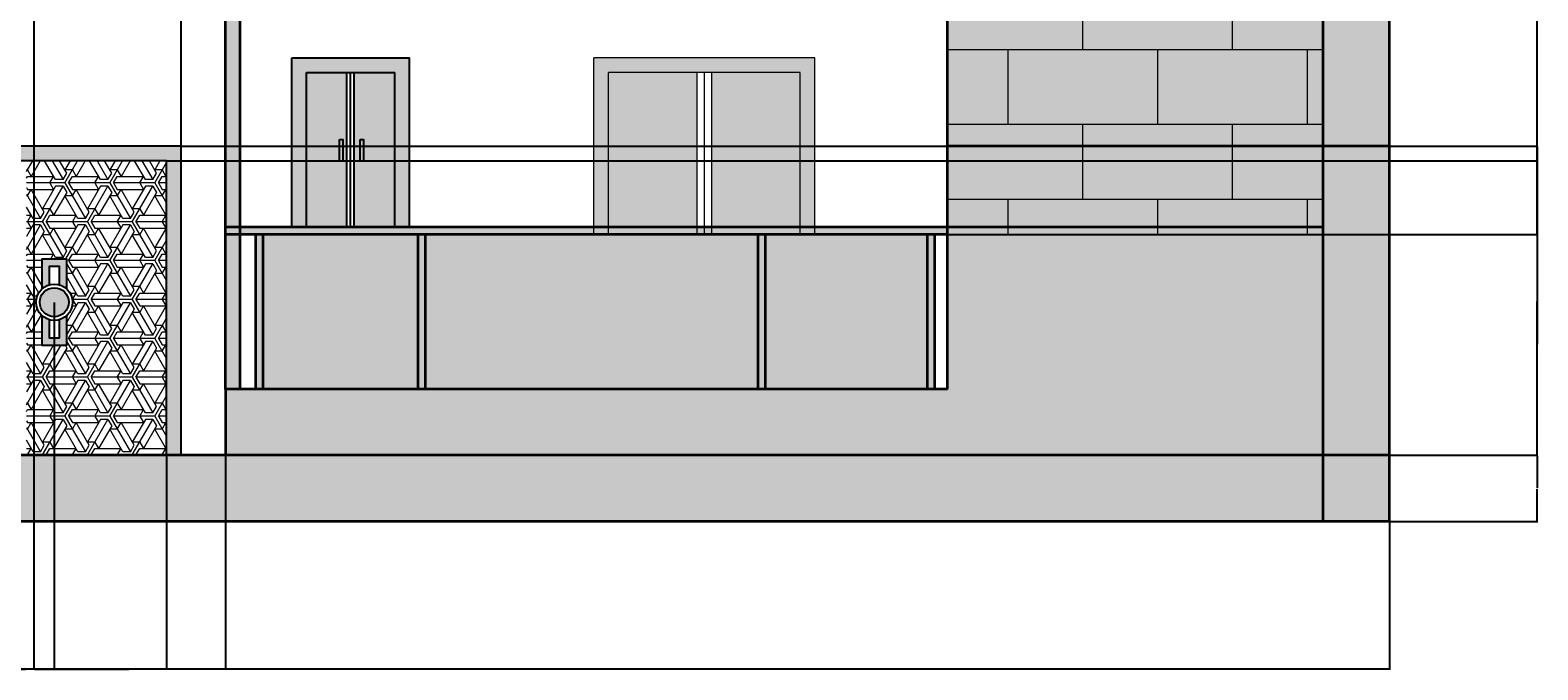
# Model space of a CAD drawing. Units: inches. Extents: x 2794 to 3619, y 522 to 1397.
# Tile 5 of 10: x 3209 to 3619, y 522 to 696. Entities that reach past the tile are written whole.
import ezdxf

# ---------------------------------------------------------------- set-up
doc = ezdxf.new("R2010")
doc.units = ezdxf.units.IN
for name, color, linetype, lineweight in [('A-ANNO-DIMS', 2, 'Continuous', 18), ('A-DOOR', 3, 'Continuous', 25), ('A-ELEV', 7, 'Continuous', 35), ('A-ELEV-PATT', 8, 'Continuous', 13), ('A-GLAZ', 4, 'Continuous', 18)]:
    doc.layers.add(name, color=color, linetype=linetype, lineweight=lineweight)
doc.styles.get("Standard").update_dxf_attribs({"font": 'arial.ttf'})
doc.dimstyles.get("Standard").update_dxf_attribs({"dimtxt": 0.18, "dimasz": 0.18, "dimexe": 0.18, "dimexo": 0.0625, "dimgap": 0.09, "dimtad": 0, "dimtih": 1, "dimtoh": 1, "dimdec": 4, "dimzin": 0, "dimdsep": 46, "dimtxsty": 'Standard', "dimcen": 0.09, "dimadec": 0, "dimazin": 0, "dimtfac": 1, "dimtdec": 4, "dimtofl": 0, "dimtmove": 0, "dimatfit": 3, "dimfxl": 1, "dimtolj": 1, "dimtzin": 0, "dimarcsym": 0})

# ---------------------------------------------------------------- blocks, each defined once
blk = doc.blocks.new('WIN-1500')
at = {"transparency": 33554646}
h = blk.add_hatch(color=256, dxfattribs=at)
h.dxf.hatch_style = 1
h.paths.add_polyline_path([(60, 48), (0, 48), (0, 2), (4, 2), (4, 44), (56, 44), (56, 2), (60, 2)])
at = {"transparency": 33554687}
h = blk.add_hatch(color=256, dxfattribs=at)
h.dxf.hatch_style = 1
h.set_gradient(color1=(248, 246, 176), color2=(74, 13, 14), name='INVCYLINDER')
h.paths.add_polyline_path([(56, 44), (32, 44), (32, 2), (56, 2)])
h.paths.add_polyline_path([(28, 44), (4, 44), (4, 2), (28, 2)])
for p, q in [((0, 0), (0, 48)), ((60, 48), (0, 48)), ((60, 0), (60, 48)), ((56, 44), (4, 44)), ((4, 0), (4, 44)), ((28, 44), (28, 0)), ((30, 44), (30, 0)), ((32, 44), (32, 0)), ((56, 0), (56, 44))]:
    blk.add_line(p, q)
blk = doc.blocks.new('DOOR-BALCONY-DBL')
at = {"transparency": 33554628}
h = blk.add_hatch(color=256, dxfattribs=at)
h.dxf.hatch_style = 1
h.paths.add_polyline_path([(4, 42), (28, 42), (28, 0), (32, 0), (32, 46), (0, 46), (0, 0), (4, 0)])
at = {"transparency": 33554646}
h = blk.add_hatch(color=256, dxfattribs=at)
h.dxf.hatch_style = 1
h.set_gradient(color1=(255, 255, 255), color2=(147, 149, 152), name='INVCYLINDER')
h.paths.add_polyline_path([(15, 42), (4, 42), (4, 0), (15, 0)])
h = blk.add_hatch(color=256, dxfattribs=at)
h.dxf.hatch_style = 1
h.set_gradient(color1=(255, 255, 255), color2=(147, 149, 152), name='INVCYLINDER')
h.paths.add_polyline_path([(28, 42), (17, 42), (17, 0), (28, 0)])
for p, q in [((0, 0), (0, 46)), ((0, 46), (32, 46)), ((4, 46), (28, 46)), ((32, 0), (32, 46)), ((4, 0), (4, 42)), ((4, 42), (28, 42)), ((15, 0), (15, 42)), ((16, 0), (16, 42)), ((17, 0), (17, 42)), ((28, 0), (28, 42))]:
    blk.add_line(p, q)
for points in [[(12.99, 23.83), (13.93, 23.83), (13.93, 17.87), (12.99, 17.87)], [(18.59, 23.83), (19.53, 23.83), (19.53, 17.87), (18.59, 17.87)]]:
    blk.add_lwpolyline(points, close=True)
blk = doc.blocks.new('*D7')
at = {"layer": 'A-ANNO-DIMS', "color": 0, "lineweight": -2, "transparency": 16777216}
for p, q in [((2834.27, 562.57), (2834.27, 522.36)), ((3578.27, 562.57), (3578.27, 522.36)), ((2834.45, 522.54), (3205.98, 522.54)), ((3578.09, 522.54), (3206.55, 522.54))]:
    blk.add_line(p, q, dxfattribs=at)
at = {"layer": 'A-ANNO-DIMS', "color": 0, "transparency": 16777216}
for points in [[(2834.45, 522.57), (2834.45, 522.51), (2834.27, 522.54)], [(3578.09, 522.57), (3578.09, 522.51), (3578.27, 522.54)]]:
    blk.add_solid(points, dxfattribs=at)
at = {"layer": 'Defpoints', "color": 0, "transparency": 16777216}
for p in [(2834.27, 562.64), (3578.27, 562.64), (3578.27, 522.54)]:
    blk.add_point(p, dxfattribs=at)
at = {"layer": 'A-ANNO-DIMS', "color": 0, "transparency": 16777216, "insert": (3206.27, 522.54), "char_height": 0.18, "attachment_point": 5}
blk.add_mtext('\\A1;744', dxfattribs=at)
blk = doc.blocks.new('*D17')
at = {"layer": 'A-ANNO-DIMS', "color": 0, "lineweight": -2, "transparency": 16777216}
for p, q in [((3578.33, 580.64), (3618.55, 580.64)), ((3618.37, 580.46), (3618.37, 571.82)), ((3618.37, 562.82), (3618.37, 571.45)), ((3578.33, 562.64), (3618.55, 562.64))]:
    blk.add_line(p, q, dxfattribs=at)
at = {"layer": 'A-ANNO-DIMS', "color": 0, "transparency": 16777216}
for points in [[(3618.34, 580.46), (3618.4, 580.46), (3618.37, 580.64)], [(3618.34, 562.82), (3618.4, 562.82), (3618.37, 562.64)]]:
    blk.add_solid(points, dxfattribs=at)
at = {"layer": 'Defpoints', "color": 0, "transparency": 16777216}
for p in [(3578.27, 580.64), (3618.37, 580.64), (3578.27, 562.64)]:
    blk.add_point(p, dxfattribs=at)
at = {"layer": 'A-ANNO-DIMS', "color": 0, "transparency": 16777216, "insert": (3618.37, 571.64), "char_height": 0.18, "attachment_point": 5}
blk.add_mtext('\\A1;18', dxfattribs=at)
blk = doc.blocks.new('*D18')
at = {"layer": 'A-ANNO-DIMS', "color": 0, "lineweight": -2, "transparency": 16777216}
for p, q in [((3458.33, 640.64), (3618.55, 640.64)), ((3618.37, 640.46), (3618.37, 610.82)), ((3618.37, 580.82), (3618.37, 610.45)), ((3578.33, 580.64), (3618.55, 580.64))]:
    blk.add_line(p, q, dxfattribs=at)
at = {"layer": 'A-ANNO-DIMS', "color": 0, "transparency": 16777216}
for points in [[(3618.34, 640.46), (3618.4, 640.46), (3618.37, 640.64)], [(3618.34, 580.82), (3618.4, 580.82), (3618.37, 580.64)]]:
    blk.add_solid(points, dxfattribs=at)
at = {"layer": 'Defpoints', "color": 0, "transparency": 16777216}
for p in [(3458.27, 640.64), (3618.37, 640.64), (3578.27, 580.64)]:
    blk.add_point(p, dxfattribs=at)
at = {"layer": 'A-ANNO-DIMS', "color": 0, "transparency": 16777216, "insert": (3618.37, 610.64), "char_height": 0.18, "attachment_point": 5}
blk.add_mtext('\\A1;60', dxfattribs=at)
blk = doc.blocks.new('*D19')
at = {"layer": 'A-ANNO-DIMS', "color": 0, "lineweight": -2, "transparency": 16777216}
for p, q in [((3458.33, 774.64), (3618.55, 774.64)), ((3618.37, 774.46), (3618.37, 707.82)), ((3618.37, 640.82), (3618.37, 707.45)), ((3458.33, 640.64), (3618.55, 640.64))]:
    blk.add_line(p, q, dxfattribs=at)
at = {"layer": 'A-ANNO-DIMS', "color": 0, "transparency": 16777216}
for points in [[(3618.34, 774.46), (3618.4, 774.46), (3618.37, 774.64)], [(3618.34, 640.82), (3618.4, 640.82), (3618.37, 640.64)]]:
    blk.add_solid(points, dxfattribs=at)
at = {"layer": 'Defpoints', "color": 0, "transparency": 16777216}
for p in [(3458.27, 774.64), (3618.37, 774.64), (3458.27, 640.64)]:
    blk.add_point(p, dxfattribs=at)
at = {"layer": 'A-ANNO-DIMS', "color": 0, "transparency": 16777216, "insert": (3618.37, 707.64), "char_height": 0.18, "attachment_point": 5}
blk.add_mtext('\\A1;134', dxfattribs=at)
blk = doc.blocks.new('*D51')
at = {"layer": 'A-ANNO-DIMS', "color": 0, "lineweight": -2, "transparency": 16777216}
for p, q in [((3206.27, 1254.57), (3206.27, 522.36)), ((3210.27, 1254.57), (3210.27, 522.36)), ((3206.45, 522.54), (3208.11, 522.54)), ((3210.09, 522.54), (3208.42, 522.54))]:
    blk.add_line(p, q, dxfattribs=at)
at = {"layer": 'A-ANNO-DIMS', "color": 0, "transparency": 16777216}
for points in [[(3206.45, 522.57), (3206.45, 522.51), (3206.27, 522.54)], [(3210.09, 522.57), (3210.09, 522.51), (3210.27, 522.54)]]:
    blk.add_solid(points, dxfattribs=at)
at = {"layer": 'Defpoints', "color": 0, "transparency": 16777216}
for p in [(3206.27, 1254.64), (3210.27, 1254.64), (3210.27, 522.54)]:
    blk.add_point(p, dxfattribs=at)
at = {"layer": 'A-ANNO-DIMS', "color": 0, "transparency": 16777216, "insert": (3208.27, 522.54), "char_height": 0.18, "attachment_point": 5}
blk.add_mtext('\\A1;4', dxfattribs=at)
blk = doc.blocks.new('*D52')
at = {"layer": 'A-ANNO-DIMS', "color": 0, "lineweight": -2, "transparency": 16777216}
for p, q in [((3210.27, 1254.57), (3210.27, 522.36)), ((3262.27, 1254.57), (3262.27, 522.36)), ((3210.45, 522.54), (3236.05, 522.54)), ((3262.09, 522.54), (3236.48, 522.54))]:
    blk.add_line(p, q, dxfattribs=at)
at = {"layer": 'A-ANNO-DIMS', "color": 0, "transparency": 16777216}
for points in [[(3210.45, 522.57), (3210.45, 522.51), (3210.27, 522.54)], [(3262.09, 522.57), (3262.09, 522.51), (3262.27, 522.54)]]:
    blk.add_solid(points, dxfattribs=at)
at = {"layer": 'Defpoints', "color": 0, "transparency": 16777216}
for p in [(3210.27, 1254.64), (3262.27, 1254.64), (3262.27, 522.54)]:
    blk.add_point(p, dxfattribs=at)
at = {"layer": 'A-ANNO-DIMS', "color": 0, "transparency": 16777216, "insert": (3236.27, 522.54), "char_height": 0.18, "attachment_point": 5}
blk.add_mtext('\\A1;52', dxfattribs=at)
blk = doc.blocks.new('*D56')
at = {"layer": 'A-ANNO-DIMS', "color": 0, "lineweight": -2, "transparency": 16777216}
for p, q in [((3162.27, 664.7), (3162.27, 1396.92)), ((3162.45, 1396.74), (3206.05, 1396.74)), ((3250.09, 1396.74), (3206.49, 1396.74)), ((3250.27, 664.7), (3250.27, 1396.92))]:
    blk.add_line(p, q, dxfattribs=at)
at = {"layer": 'A-ANNO-DIMS', "color": 0, "transparency": 16777216}
for points in [[(3162.45, 1396.77), (3162.45, 1396.71), (3162.27, 1396.74)], [(3250.09, 1396.77), (3250.09, 1396.71), (3250.27, 1396.74)]]:
    blk.add_solid(points, dxfattribs=at)
at = {"layer": 'Defpoints', "color": 0, "transparency": 16777216}
for p in [(3250.27, 1396.74), (3162.27, 664.64), (3250.27, 664.64)]:
    blk.add_point(p, dxfattribs=at)
at = {"layer": 'A-ANNO-DIMS', "color": 0, "transparency": 16777216, "insert": (3206.27, 1396.74), "char_height": 0.18, "attachment_point": 5}
blk.add_mtext('\\A1;88', dxfattribs=at)
blk = doc.blocks.new('*D59')
at = {"layer": 'A-ANNO-DIMS', "color": 0, "lineweight": -2, "transparency": 16777216}
for p, q in [((3250.33, 664.64), (3618.55, 664.64)), ((3618.37, 664.46), (3618.37, 622.82)), ((3618.37, 580.82), (3618.37, 622.45)), ((3250.33, 580.64), (3618.55, 580.64))]:
    blk.add_line(p, q, dxfattribs=at)
at = {"layer": 'A-ANNO-DIMS', "color": 0, "transparency": 16777216}
for points in [[(3618.34, 664.46), (3618.4, 664.46), (3618.37, 664.64)], [(3618.34, 580.82), (3618.4, 580.82), (3618.37, 580.64)]]:
    blk.add_solid(points, dxfattribs=at)
at = {"layer": 'Defpoints', "color": 0, "transparency": 16777216}
for p in [(3250.27, 664.64), (3618.37, 664.64), (3250.27, 580.64)]:
    blk.add_point(p, dxfattribs=at)
at = {"layer": 'A-ANNO-DIMS', "color": 0, "transparency": 16777216, "insert": (3618.37, 622.64), "char_height": 0.18, "attachment_point": 5}
blk.add_mtext('\\A1;84', dxfattribs=at)
blk = doc.blocks.new('*D60')
at = {"layer": 'A-ANNO-DIMS', "color": 0, "lineweight": -2, "transparency": 16777216}
for p, q in [((3250.328351, 664.635093), (3618.545851, 664.635093)), ((3618.365851, 664.455093), (3618.365851, 662.815093)), ((3246.328351, 660.635093), (3618.545851, 660.635093)), ((3618.365851, 660.815093), (3618.365851, 662.455093))]:
    blk.add_line(p, q, dxfattribs=at)
at = {"layer": 'A-ANNO-DIMS', "color": 0, "transparency": 16777216}
for points in [[(3618.335851, 664.455093), (3618.395851, 664.455093), (3618.365851, 664.635093)], [(3618.335851, 660.815093), (3618.395851, 660.815093), (3618.365851, 660.635093)]]:
    blk.add_solid(points, dxfattribs=at)
at = {"layer": 'Defpoints', "color": 0, "transparency": 16777216}
for p in [(3250.265851, 664.635093), (3246.265851, 660.635093), (3618.365851, 660.635093)]:
    blk.add_point(p, dxfattribs=at)
at = {"layer": 'A-ANNO-DIMS', "color": 0, "transparency": 16777216, "insert": (3618.365851, 662.635093), "char_height": 0.18, "attachment_point": 5}
blk.add_mtext('\\A1;4', dxfattribs=at)
blk = doc.blocks.new('*D62')
at = {"layer": 'A-ANNO-DIMS', "color": 0, "lineweight": -2, "transparency": 16777216}
for p, q in [((3215.82, 622.15), (3215.82, 522.36)), ((3246.27, 580.57), (3246.27, 522.36)), ((3216, 522.54), (3230.65, 522.54)), ((3246.09, 522.54), (3231.44, 522.54))]:
    blk.add_line(p, q, dxfattribs=at)
at = {"layer": 'A-ANNO-DIMS', "color": 0, "transparency": 16777216}
for points in [[(3216, 522.57), (3216, 522.51), (3215.82, 522.54)], [(3246.09, 522.57), (3246.09, 522.51), (3246.27, 522.54)]]:
    blk.add_solid(points, dxfattribs=at)
at = {"layer": 'Defpoints', "color": 0, "transparency": 16777216}
for p in [(3215.82, 622.22), (3246.27, 580.64), (3246.27, 522.54)]:
    blk.add_point(p, dxfattribs=at)
at = {"layer": 'A-ANNO-DIMS', "color": 0, "transparency": 16777216, "insert": (3231.04, 522.54), "char_height": 0.18, "attachment_point": 5}
blk.add_mtext('\\A1;30.45', dxfattribs=at)

msp = doc.modelspace()

# ---------------------------------------------------------------- hatches: boundary and pattern name
at = {"layer": 'A-ELEV-PATT', "transparency": 33554687}
h = msp.add_hatch(color=256, dxfattribs=at)
h.dxf.hatch_style = 1
h.paths.add_polyline_path([(3578.2659, 1294.6351), (3560.2659, 1294.6351), (3560.2659, 642.6351), (3578.2659, 642.6351)])
h.paths.add_polyline_path([(2852.2659, 1294.6351), (2834.2659, 1294.6351), (2834.2659, 642.6351), (2852.2659, 642.6351)])
h = msp.add_hatch(color=256, dxfattribs=at)
h.dxf.hatch_style = 1
h.paths.add_polyline_path([(2852.2659, 1294.6351), (2834.2659, 1294.6351), (2834.2659, 562.6351), (2852.2659, 562.6351)])
h.paths.add_polyline_path([(3578.2659, 1294.6351), (3560.2659, 1294.6351), (3560.2659, 562.6351), (3578.2659, 562.6351)])
at = {"layer": 'A-ELEV-PATT'}
h = msp.add_hatch(dxfattribs=at)
h.set_pattern_fill('AR-B816', color=256, scale=0.1)
h.paths.add_polyline_path([(2954.2659, 1114.6351), (2852.2659, 1114.6351), (2852.2659, 994.6351), (2954.2659, 994.6351)])
h.paths.add_polyline_path([(2954.2659, 1246.6351), (2852.2659, 1246.6351), (2852.2659, 1126.6351), (2954.2659, 1126.6351)])
h.paths.add_polyline_path([(2954.2659, 982.6351), (2852.2659, 982.6351), (2852.2659, 862.6351), (2954.2659, 862.6351)])
h.paths.add_polyline_path([(2954.2659, 850.6351), (2852.2659, 850.6351), (2852.2659, 730.6351), (2954.2659, 730.6351)])
h.paths.add_polyline_path([(3560.2659, 850.6351), (3458.2659, 850.6351), (3458.2659, 730.6351), (3560.2659, 730.6351)])
h.paths.add_polyline_path([(3560.2659, 982.6351), (3458.2659, 982.6351), (3458.2659, 862.6351), (3560.2659, 862.6351)])
h.paths.add_polyline_path([(3560.2659, 1114.6351), (3458.2659, 1114.6351), (3458.2659, 994.6351), (3560.2659, 994.6351)])
h.paths.add_polyline_path([(3560.2659, 1246.6351), (3458.2659, 1246.6351), (3458.2659, 1126.6351), (3560.2659, 1126.6351)])
h.paths.add_polyline_path([(2852.2659, 642.6351), (2954.2659, 642.6351), (2954.2659, 718.6351), (2852.2659, 718.6351)])
h.paths.add_polyline_path([(3458.2659, 640.6351), (3560.2659, 640.6351), (3560.2659, 718.6351), (3458.2659, 718.6351)])
at = {"layer": 'A-ELEV-PATT', "transparency": 33554630}
h = msp.add_hatch(color=256, dxfattribs=at)
h.dxf.hatch_style = 1
h.paths.add_polyline_path([(2954.2659, 1114.6351), (2852.2659, 1114.6351), (2852.2659, 994.6351), (2954.2659, 994.6351)])
h.paths.add_polyline_path([(2954.2659, 982.6351), (2852.2659, 982.6351), (2852.2659, 862.6351), (2954.2659, 862.6351)])
h.paths.add_polyline_path([(2954.2659, 850.6351), (2852.2659, 850.6351), (2852.2659, 730.6351), (2954.2659, 730.6351)])
h.paths.add_polyline_path([(3560.2659, 850.6351), (3458.2659, 850.6351), (3458.2659, 730.6351), (3560.2659, 730.6351)])
h.paths.add_polyline_path([(3560.2659, 982.6351), (3458.2659, 982.6351), (3458.2659, 862.6351), (3560.2659, 862.6351)])
h.paths.add_polyline_path([(3560.2659, 1114.6351), (3458.2659, 1114.6351), (3458.2659, 994.6351), (3560.2659, 994.6351)])
h.paths.add_polyline_path([(3560.2659, 1246.6351), (3458.2659, 1246.6351), (3458.2659, 1126.6351), (3560.2659, 1126.6351)])
h.paths.add_polyline_path([(2852.2659, 642.6351), (2954.2659, 642.6351), (2954.2659, 718.6351), (2852.2659, 718.6351)])
h.paths.add_polyline_path([(3458.2659, 642.6351), (3560.2659, 642.6351), (3560.2659, 718.6351), (3458.2659, 718.6351)])
at = {"layer": 'A-ELEV-PATT', "transparency": 33554687}
h = msp.add_hatch(color=256, dxfattribs=at)
h.dxf.hatch_style = 1
h.paths.add_polyline_path([(3266.2659, 700.6351), (3262.2659, 700.6351), (3262.2659, 642.6351), (3266.2659, 642.6351)])
h.paths.add_polyline_path([(3266.2659, 640.6351), (3262.2659, 640.6351), (3262.2659, 598.6351), (3266.2659, 598.6351)])
h.paths.add_polyline_path([(3458.2659, 642.6351), (3266.2659, 642.6351), (3266.2659, 640.6351), (3458.2659, 640.6351)])
h.paths.add_polyline_path([(3272.4761, 640.6351), (3270.4761, 640.6351), (3270.4761, 598.6351), (3272.4761, 598.6351)])
h.paths.add_polyline_path([(3316.4761, 640.6351), (3314.4761, 640.6351), (3314.4761, 598.6351), (3316.4761, 598.6351)])
h.paths.add_polyline_path([(3266.2659, 642.6351), (3262.2659, 642.6351), (3262.2659, 640.6351), (3266.2659, 640.6351)])
h.paths.add_polyline_path([(3150.2659, 640.6351), (3146.2659, 640.6351), (3146.2659, 598.6351), (3150.2659, 598.6351)])
h = msp.add_hatch(color=256, dxfattribs=at)
h.dxf.hatch_style = 1
h.paths.add_polyline_path([(3246.2659, 664.6351), (3166.2659, 664.6351), (3166.2659, 660.6351), (3246.2659, 660.6351)])
h.paths.add_polyline_path([(3166.2659, 660.6351), (3162.2659, 660.6351), (3162.2659, 580.6351), (3166.2659, 580.6351)])
h.paths.add_polyline_path([(3250.2659, 660.6351), (3246.2659, 660.6351), (3246.2659, 580.6351), (3250.2659, 580.6351)])
h = msp.add_hatch(color=256, dxfattribs=at)
h.dxf.hatch_style = 1
h.paths.add_polyline_path([(3166.2659, 664.6351), (3162.2659, 664.6351), (3162.2659, 660.6351), (3166.2659, 660.6351)])
h.paths.add_polyline_path([(3250.2659, 664.6351), (3246.2659, 664.6351), (3246.2659, 660.6351), (3250.2659, 660.6351)])
h = msp.add_hatch(dxfattribs=at)
h.set_pattern_fill('ESCHER', color=256, scale=0.4)
h.paths.add_polyline_path([(3204.2659, 660.6351), (3166.2659, 660.6351), (3166.2659, 580.6351), (3204.2659, 580.6351)])
h.paths.add_polyline_path([(3192.5875, 634.0076), (3199.1979, 634.0076), (3199.1979, 625.8832, -0.21239083), (3200.8288, 622.217, -0.21239083), (3199.1979, 618.5509), (3199.1979, 610.4265), (3192.5875, 610.4265), (3192.5875, 618.5509, -0.21239083), (3190.9566, 622.217, -0.21239083), (3192.5875, 625.8832)], flags=16)
h.paths.add_polyline_path([(3199.8288, 622.217, -1), (3191.9566, 622.217, -1)], flags=0)
h.paths.add_polyline_path([(3246.2659, 660.6351), (3208.2659, 660.6351), (3208.2659, 580.6351), (3246.2659, 580.6351)])
h.paths.add_polyline_path([(3219.1237, 634.0076), (3219.1237, 625.8832, -0.21239083), (3220.7546, 622.217, -0.21239083), (3219.1237, 618.5509), (3219.1237, 610.4265), (3212.5133, 610.4265), (3212.5133, 618.5509, -0.21239083), (3210.8824, 622.217, -0.21239083), (3212.5133, 625.8832), (3212.5133, 634.0076)], flags=16)
h.paths.add_polyline_path([(3219.7546, 622.217, -1), (3211.8824, 622.217, -1)], flags=0)
h = msp.add_hatch(color=256, dxfattribs=at)
h.dxf.hatch_style = 1
h.paths.add_polyline_path([(2954.2659, 642.6351), (2852.2659, 642.6351), (2852.2659, 598.6351), (2954.2659, 598.6351)])
h.paths.add_polyline_path([(3150.2659, 598.6351), (2852.2659, 598.6351), (2852.2659, 580.6351), (3150.2659, 580.6351)])
h.paths.add_polyline_path([(3560.2659, 642.6351), (3458.2659, 642.6351), (3458.2659, 598.6351), (3560.2659, 598.6351)])
h.paths.add_polyline_path([(3560.2659, 598.6351), (3262.2659, 598.6351), (3262.2659, 580.6351), (3560.2659, 580.6351)])
h = msp.add_hatch(color=256, dxfattribs=at)
h.dxf.hatch_style = 1
h.paths.add_polyline_path([(3142.3604, 640.6351), (3140.3604, 640.6351), (3140.3604, 598.6351), (3142.3604, 598.6351)])
h.paths.add_polyline_path([(3146.2659, 642.6351), (2954.2659, 642.6351), (2954.2659, 640.6351), (3146.2659, 640.6351)])
h.paths.add_polyline_path([(3096.3813, 640.6351), (3094.3813, 640.6351), (3094.3813, 598.6351), (3096.3813, 598.6351)])
h.paths.add_polyline_path([(3004.0752, 640.6351), (3002.0752, 640.6351), (3002.0752, 598.6351), (3004.0752, 598.6351)])
h.paths.add_polyline_path([(2960.0752, 640.6351), (2958.0752, 640.6351), (2958.0752, 598.6351), (2960.0752, 598.6351)])
h.paths.add_polyline_path([(3408.7822, 640.6351), (3406.7822, 640.6351), (3406.7822, 598.6351), (3408.7822, 598.6351)])
h.paths.add_polyline_path([(3454.7613, 640.6351), (3452.7613, 640.6351), (3452.7613, 598.6351), (3454.7613, 598.6351)])
h = msp.add_hatch(dxfattribs=at)
h.set_pattern_fill('EARTH', color=256)
h.paths.add_polyline_path([(3002.0752, 640.6351), (2960.0752, 640.6351), (2960.0752, 598.6351), (3002.0752, 598.6351)])
h.paths.add_polyline_path([(3094.3813, 640.6351), (3004.0752, 640.6351), (3004.0752, 598.6351), (3094.3813, 598.6351)])
h.paths.add_polyline_path([(3140.3604, 640.6351), (3096.3813, 640.6351), (3096.3813, 598.6351), (3140.3604, 598.6351)])
h.paths.add_polyline_path([(3314.4761, 640.6351), (3272.4761, 640.6351), (3272.4761, 598.6351), (3314.4761, 598.6351)])
h.paths.add_polyline_path([(3406.7822, 640.6351), (3316.4761, 640.6351), (3316.4761, 598.6351), (3406.7822, 598.6351)])
h.paths.add_polyline_path([(3452.7613, 640.6351), (3408.7822, 640.6351), (3408.7822, 598.6351), (3452.7613, 598.6351)])
h = msp.add_hatch(color=256, dxfattribs=at)
h.dxf.hatch_style = 1
h.paths.add_polyline_path([(3199.1979, 634.0076), (3192.5875, 634.0076), (3192.5875, 625.8832, -0.11704667), (3194.5875, 626.9774), (3194.5875, 632.0076), (3197.1979, 632.0076), (3197.1979, 626.9774, -0.11704667), (3199.1979, 625.8832)])
h.paths.add_polyline_path([(3199.1979, 618.5509, -0.11704667), (3197.1979, 617.4566), (3197.1979, 612.4265), (3194.5875, 612.4265), (3194.5875, 617.4566, -0.11704667), (3192.5875, 618.5509), (3192.5875, 610.4265), (3199.1979, 610.4265)])
h.paths.add_polyline_path([(3191.9566, 622.217, 1), (3199.8288, 622.217, 1)])
h.paths.add_polyline_path([(3219.1237, 634.0076), (3212.5133, 634.0076), (3212.5133, 625.8832, -0.11704667), (3214.5133, 626.9774), (3214.5133, 632.0076), (3217.1237, 632.0076), (3217.1237, 626.9774, -0.11704667), (3219.1237, 625.8832)])
h.paths.add_polyline_path([(3219.1237, 618.5509, -0.11704667), (3217.1237, 617.4566), (3217.1237, 612.4265), (3214.5133, 612.4265), (3214.5133, 617.4566, -0.11704667), (3212.5133, 618.5509), (3212.5133, 610.4265), (3219.1237, 610.4265)])
h.paths.add_polyline_path([(3211.8824, 622.217, 1), (3219.7546, 622.217, 1)])
h = msp.add_hatch(color=256, dxfattribs=at)
h.dxf.hatch_style = 1
h.paths.add_polyline_path([(3560.2659, 580.6351), (2852.2659, 580.6351), (2852.2659, 562.6351), (3560.2659, 562.6351)])

# ---------------------------------------------------------------- linework, layer by layer
at = {"layer": 'A-DOOR'}
for p, q in [((3250.2659, 664.6351), (3162.2659, 664.6351)), ((3250.2659, 580.6351), (3250.2659, 664.6351)), ((3246.2659, 660.6351), (3166.2659, 660.6351)), ((3246.2659, 580.6351), (3246.2659, 660.6351))]:
    msp.add_line(p, q, dxfattribs=at)
for points in [[(3212.5133, 625.8832), (3212.5133, 634.0076), (3219.1237, 634.0076), (3219.1237, 625.8832)], [(3214.5133, 626.9774), (3214.5133, 632.0076), (3217.1237, 632.0076), (3217.1237, 626.9774)], [(3219.1237, 618.5509), (3219.1237, 610.4265), (3212.5133, 610.4265), (3212.5133, 618.5509)], [(3217.1237, 617.4566), (3217.1237, 612.4265), (3214.5133, 612.4265), (3214.5133, 617.4566)]]:
    msp.add_lwpolyline(points, dxfattribs=at)
for radius in [4.9361, 3.9361]:
    msp.add_circle((3215.8185, 622.217), radius, dxfattribs=at)
at = {"layer": 'A-ELEV'}
for p, q in [((3578.2659, 562.6351), (3578.2659, 1297.6351)), ((3458.2659, 598.6351), (3458.2659, 1294.6351)), ((3560.2659, 562.6351), (3560.2659, 1294.6351)), ((3262.2659, 598.6351), (3262.2659, 1258.6351)), ((3266.2659, 598.6351), (3266.2659, 1258.6351)), ((3578.2659, 664.6351), (3458.2659, 664.6351)), ((3560.2659, 642.6351), (3262.2659, 642.6351)), ((3458.2659, 640.6351), (3262.2659, 640.6351)), ((3270.4761, 640.6351), (3270.4761, 598.6351)), ((3272.4761, 640.6351), (3272.4761, 598.6351)), ((3314.4761, 640.6351), (3314.4761, 598.6351)), ((3316.4761, 640.6351), (3316.4761, 598.6351)), ((3406.7822, 640.6351), (3406.7822, 598.6351)), ((3408.7822, 640.6351), (3408.7822, 598.6351)), ((3452.7613, 640.6351), (3452.7613, 598.6351)), ((3454.7613, 640.6351), (3454.7613, 598.6351)), ((3458.2659, 598.6351), (3262.2659, 598.6351)), ((3262.2659, 598.6351), (3262.2659, 580.6351)), ((3578.2659, 580.6351), (2834.2659, 580.6351)), ((3578.2659, 562.6351), (2834.2659, 562.6351))]:
    msp.add_line(p, q, dxfattribs=at)

# ---------------------------------------------------------------- block references
at = {"layer": 'A-DOOR'}
msp.add_blockref('DOOR-BALCONY-DBL', (3280.266, 642.635), dxfattribs=at)
at = {"layer": 'A-GLAZ'}
msp.add_blockref('WIN-1500', (3362.266, 640.635), dxfattribs=at)

# ---------------------------------------------------------------- dimensions: what is measured, and where the dimension line sits
at = {"layer": 'A-ANNO-DIMS'}
for base, p1, p2, override, picture, middle in [((3250.2659, 1396.7351), (3162.2659, 664.6351), (3250.2659, 664.6351), {"dimdec": 0, "dimlfac": 1, "dimrnd": 0, "dimzin": 0, "dimdsep": 46, "dimlunit": 2}, '*D56', (3206.2659, 1396.7351)), ((3210.2659, 522.5351), (3206.2659, 1254.6351), (3210.2659, 1254.6351), {"dimdec": 0, "dimlfac": 1, "dimrnd": 0, "dimzin": 0, "dimdsep": 46, "dimlunit": 2}, '*D51', (3208.2659, 522.5351)), ((3262.2659, 522.5351), (3210.2659, 1254.6351), (3262.2659, 1254.6351), {"dimdec": 0, "dimlfac": 1, "dimrnd": 0, "dimzin": 0, "dimdsep": 46, "dimlunit": 2}, '*D52', (3236.2659, 522.5351)), ((3246.2659, 522.5351), (3215.8185, 622.217), (3246.2659, 580.6351), {"dimdec": 2, "dimlfac": 1, "dimrnd": 0, "dimzin": 0, "dimdsep": 46, "dimlunit": 2}, '*D62', (3231.0422, 522.5351)), ((3578.2659, 522.5351), (2834.2659, 562.6351), (3578.2659, 562.6351), {"dimdec": 0, "dimlfac": 1, "dimrnd": 0, "dimzin": 0, "dimdsep": 46, "dimlunit": 2}, '*D7', (3206.2659, 522.5351))]:
    dim = msp.add_linear_dim(base=base, p1=p1, p2=p2, dimstyle='Standard', override=override, dxfattribs=at)
    dim.commit()
    dim.dimension.update_dxf_attribs({"geometry": picture, "text_midpoint": middle})
for base, p1, p2, picture, middle in [((3618.3659, 774.6351), (3458.2659, 640.6351), (3458.2659, 774.6351), '*D19', (3618.3659, 707.6351)), ((3618.3659, 660.6351), (3250.2659, 664.6351), (3246.2659, 660.6351), '*D60', (3618.3659, 662.6351)), ((3618.3659, 664.6351), (3250.2659, 580.6351), (3250.2659, 664.6351), '*D59', (3618.3659, 622.6351)), ((3618.3659, 640.6351), (3578.2659, 580.6351), (3458.2659, 640.6351), '*D18', (3618.3659, 610.6351)), ((3618.3659, 580.6351), (3578.2659, 562.6351), (3578.2659, 580.6351), '*D17', (3618.3659, 571.6351))]:
    dim = msp.add_linear_dim(base=base, p1=p1, p2=p2, angle=90, dimstyle='Standard', override={"dimdec": 0, "dimlfac": 1, "dimrnd": 0, "dimzin": 0, "dimdsep": 46, "dimlunit": 2}, dxfattribs=at)
    dim.commit()
    dim.dimension.update_dxf_attribs({"geometry": picture, "text_midpoint": middle})

doc.saveas('drawing.dxf')
